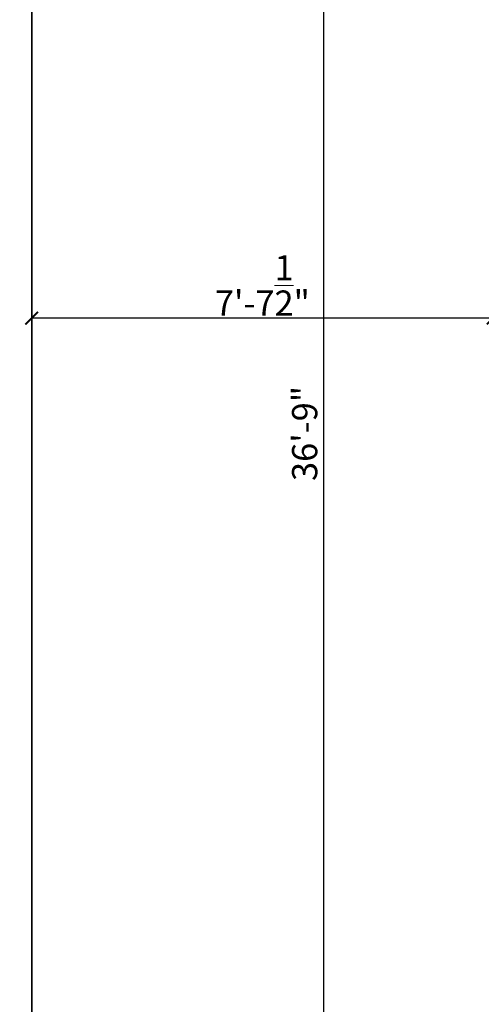
# Model space of a CAD drawing. Units: inches. Extents: x 3283068 to 3284536, y 3240756 to 3241803.
# Tile 4 of 19: x 3283246 to 3283337, y 3241305 to 3241501. Entities that reach past the tile are written whole.
import ezdxf

# ---------------------------------------------------------------- set-up
doc = ezdxf.new("R2010")
doc.units = ezdxf.units.IN
doc.layers.add('A-ANNO-DIMS', color=2, linetype='Continuous', lineweight=18)
doc.layers.add('C-PROP', color=7, linetype='Continuous', lineweight=25)
doc.styles.get("Standard").update_dxf_attribs({"font": 'arial.ttf'})
doc.dimstyles.new('ISO-25', dxfattribs={"dimtxt": 5, "dimasz": 2.5, "dimexe": 1.25, "dimexo": 0.625, "dimtad": 1, "dimlunit": 4, "dimtxsty": 'Standard', "dimblk": 'ARCHTICK', "dimcen": 2.5, "dimadec": 0, "dimazin": 0, "dimtfac": 1, "dimtmove": 0, "dimatfit": 3, "dimfxl": 1, "dimarcsym": 0})

# ---------------------------------------------------------------- blocks, each defined once
blk = doc.blocks.new('_ArchTick')
at = {"color": 0, "linetype": 'ByBlock', "const_width": 0.15}
blk.add_lwpolyline([(-0.5, -0.5), (0.5, 0.5)], dxfattribs=at)
blk = doc.blocks.new('*D1')
at = {"layer": 'A-ANNO-DIMS', "color": 0, "lineweight": -2, "transparency": 16777216}
for p, q in [((3283338.96, 3241639.1), (3283304.8, 3241639.1)), ((3283306.05, 3241198.1), (3283306.05, 3241639.1)), ((3283338.96, 3241198.1), (3283304.8, 3241198.1))]:
    blk.add_line(p, q, dxfattribs=at)
at = {"layer": 'Defpoints', "color": 0, "transparency": 16777216}
for p in [(3283306.05, 3241639.1), (3283339.59, 3241639.1), (3283339.59, 3241198.1)]:
    blk.add_point(p, dxfattribs=at)
at = {"layer": 'A-ANNO-DIMS', "color": 0, "lineweight": -2, "transparency": 16777216, "xscale": 2.5, "yscale": 2.5, "zscale": 2.5}
for p, rotation in [((3283306.05, 3241639.1), 90), ((3283306.05, 3241198.1), 270)]:
    blk.add_blockref('_ArchTick', p, dxfattribs=dict(at, rotation=rotation))
at = {"layer": 'A-ANNO-DIMS', "color": 0, "transparency": 16777216, "insert": (3283302.87, 3241418.6), "char_height": 5, "attachment_point": 5, "rotation": 90}
blk.add_mtext('36\'-9"', dxfattribs=at)
blk = doc.blocks.new('*D26')
at = {"layer": 'A-ANNO-DIMS', "color": 0, "lineweight": -2, "transparency": 16777216}
for p, q in [((3283248.09, 3241434.23), (3283248.09, 3241442.74)), ((3283339.59, 3241441.49), (3283248.09, 3241441.49)), ((3283339.59, 3241434.23), (3283339.59, 3241442.74))]:
    blk.add_line(p, q, dxfattribs=at)
at = {"layer": 'Defpoints', "color": 0, "transparency": 16777216}
for p in [(3283248.09, 3241441.49), (3283248.09, 3241433.6), (3283339.59, 3241433.6)]:
    blk.add_point(p, dxfattribs=at)
at = {"layer": 'A-ANNO-DIMS', "color": 0, "lineweight": -2, "transparency": 16777216, "xscale": 2.5, "yscale": 2.5, "zscale": 2.5, "rotation": 180}
blk.add_blockref('_ArchTick', (3283248.09, 3241441.49), dxfattribs=at)
at = {"layer": 'A-ANNO-DIMS', "color": 0, "lineweight": -2, "transparency": 16777216, "xscale": 2.5, "yscale": 2.5, "zscale": 2.5}
blk.add_blockref('_ArchTick', (3283339.59, 3241441.49), dxfattribs=at)
at = {"layer": 'A-ANNO-DIMS', "color": 0, "transparency": 16777216, "insert": (3283293.84, 3241447.97), "char_height": 5, "attachment_point": 5}
blk.add_mtext('7\'-7{\\H1x;\\S1/2;}"', dxfattribs=at)
blk = doc.blocks.new('*D61')
at = {"layer": 'A-ANNO-DIMS', "color": 0, "lineweight": -2, "transparency": 16777216}
for p, q in [((3283247.46, 3241730.6), (3283073.57, 3241730.6)), ((3283074.82, 3241082.6), (3283074.82, 3241730.6)), ((3283247.46, 3241082.6), (3283073.57, 3241082.6))]:
    blk.add_line(p, q, dxfattribs=at)
at = {"layer": 'Defpoints', "color": 0, "transparency": 16777216}
for p in [(3283074.82, 3241730.6), (3283248.09, 3241730.6), (3283248.09, 3241082.6)]:
    blk.add_point(p, dxfattribs=at)
at = {"layer": 'A-ANNO-DIMS', "color": 0, "lineweight": -2, "transparency": 16777216, "xscale": 2.5, "yscale": 2.5, "zscale": 2.5}
for p, rotation in [((3283074.82, 3241730.6), 90), ((3283074.82, 3241082.6), 270)]:
    blk.add_blockref('_ArchTick', p, dxfattribs=dict(at, rotation=rotation))
at = {"layer": 'A-ANNO-DIMS', "color": 0, "transparency": 16777216, "insert": (3283071.64, 3241406.6), "char_height": 5, "attachment_point": 5, "rotation": 90}
blk.add_mtext('54\'-0"', dxfattribs=at)
blk = doc.blocks.new('*D63')
at = {"layer": 'A-ANNO-DIMS', "color": 0, "lineweight": -2, "transparency": 16777216}
for p, q in [((3283248.09, 3241083.23), (3283248.09, 3241798.08)), ((3283248.09, 3241796.83), (3284328.09, 3241796.83)), ((3284328.09, 3241083.23), (3284328.09, 3241798.08))]:
    blk.add_line(p, q, dxfattribs=at)
at = {"layer": 'Defpoints', "color": 0, "transparency": 16777216}
for p in [(3284328.09, 3241796.83), (3283248.09, 3241082.6), (3284328.09, 3241082.6)]:
    blk.add_point(p, dxfattribs=at)
at = {"layer": 'A-ANNO-DIMS', "color": 0, "lineweight": -2, "transparency": 16777216, "xscale": 2.5, "yscale": 2.5, "zscale": 2.5, "rotation": 180}
blk.add_blockref('_ArchTick', (3283248.09, 3241796.83), dxfattribs=at)
at = {"layer": 'A-ANNO-DIMS', "color": 0, "lineweight": -2, "transparency": 16777216, "xscale": 2.5, "yscale": 2.5, "zscale": 2.5}
blk.add_blockref('_ArchTick', (3284328.09, 3241796.83), dxfattribs=at)
at = {"layer": 'A-ANNO-DIMS', "color": 0, "transparency": 16777216, "insert": (3283788.09, 3241800.01), "char_height": 5, "attachment_point": 5}
blk.add_mtext('90\'-0"', dxfattribs=at)

msp = doc.modelspace()

# ---------------------------------------------------------------- linework, layer by layer
at = {"layer": 'C-PROP'}
msp.add_line((3283248.089, 3241730.602), (3283248.089, 3241082.602), dxfattribs=at)

# ---------------------------------------------------------------- dimensions: what is measured, and where the dimension line sits
at = {"layer": 'A-ANNO-DIMS'}
for base, p1, p2, override, picture, middle in [((3284328.089, 3241796.827), (3283248.089, 3241082.602), (3284328.089, 3241082.602), {"dimdec": 1, "dimlfac": 1, "dimrnd": 0, "dimzin": 1, "dimdsep": 46, "dimlunit": 4, "dimfrac": 2}, '*D63', (3283788.089, 3241800.005)), ((3283248.089, 3241441.495), (3283339.589, 3241433.602), (3283248.089, 3241433.602), {"dimclrd": 0, "dimclre": 0, "dimclrt": 0}, '*D26', (3283293.839, 3241447.974))]:
    dim = msp.add_linear_dim(base=base, p1=p1, p2=p2, dimstyle='ISO-25', override=override, dxfattribs=at)
    dim.commit()
    dim.dimension.update_dxf_attribs({"geometry": picture, "text_midpoint": middle})
for base, p1, p2, override, picture, middle in [((3283074.817, 3241730.602), (3283248.089, 3241082.602), (3283248.089, 3241730.602), {"dimdec": 1, "dimlfac": 1, "dimrnd": 0, "dimzin": 1, "dimdsep": 46, "dimlunit": 4, "dimfrac": 2}, '*D61', (3283071.639, 3241406.602)), ((3283306.051, 3241639.102), (3283339.589, 3241198.102), (3283339.589, 3241639.102), {"dimclrd": 0, "dimclre": 0, "dimclrt": 0}, '*D1', (3283302.872, 3241418.602))]:
    dim = msp.add_linear_dim(base=base, p1=p1, p2=p2, angle=90, dimstyle='ISO-25', override=override, dxfattribs=at)
    dim.commit()
    dim.dimension.update_dxf_attribs({"geometry": picture, "text_midpoint": middle})

doc.saveas('drawing.dxf')
